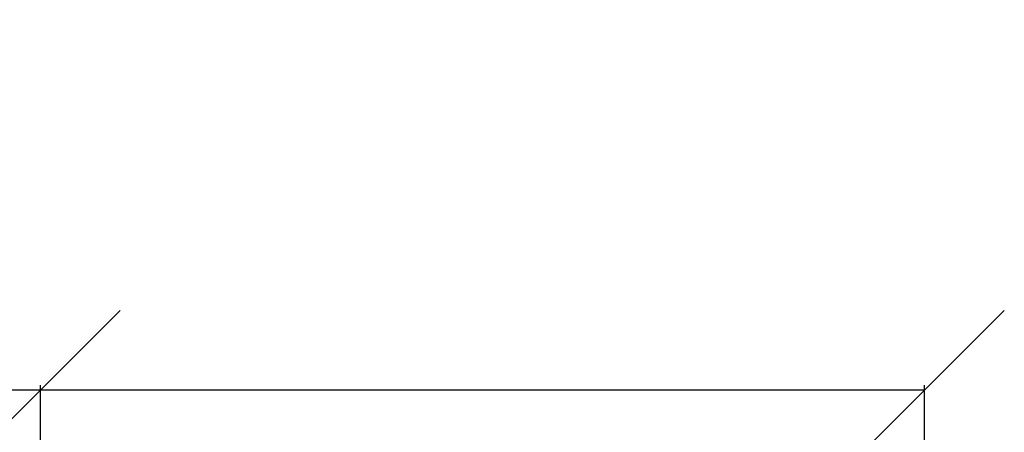
# Model space of a CAD drawing. Units: inches. Extents: x -1198 to -69, y -512 to 437.
# Tile 15 of 50: x -979 to -942, y 189 to 204. Entities that reach past the tile are written whole.
import ezdxf

# ---------------------------------------------------------------- set-up
doc = ezdxf.new("R2010")
doc.units = ezdxf.units.IN
doc.header["$MEASUREMENT"] = 0
doc.layers.add('A-ANNO-DIMS', color=2, linetype='Continuous', lineweight=18)
doc.styles.get("Standard").update_dxf_attribs({"font": 'arial.ttf'})
doc.dimstyles.get("Standard").update_dxf_attribs({"dimtxt": 6, "dimasz": 6, "dimexe": 0.18, "dimexo": 0.0625, "dimgap": 0.09, "dimtad": 0, "dimtih": 1, "dimtoh": 1, "dimdec": 0, "dimzin": 0, "dimdsep": 46, "dimlunit": 4, "dimtxsty": 'Standard', "dimblk": 'OBLIQUE', "dimcen": 0.09, "dimadec": 0, "dimazin": 0, "dimtfac": 1, "dimtdec": 0, "dimtofl": 0, "dimtmove": 0, "dimatfit": 3, "dimfxl": 1, "dimtolj": 1, "dimtzin": 0, "dimarcsym": 0})

# ---------------------------------------------------------------- blocks, each defined once
blk = doc.blocks.new('_Oblique')
at = {"color": 0, "linetype": 'ByBlock', "lineweight": -2}
blk.add_line((-0.5, -0.5), (0.5, 0.5), dxfattribs=at)
blk = doc.blocks.new('*D50')
at = {"layer": 'A-ANNO-DIMS', "color": 0, "lineweight": -2, "ltscale": 10, "transparency": 16777216}
for p, q in [((-978.462, 185.29), (-978.462, 190.403)), ((-945.163, 185.29), (-945.163, 190.403)), ((-978.462, 190.223), (-984.462, 190.223)), ((-945.163, 190.223), (-978.462, 190.223))]:
    blk.add_line(p, q, dxfattribs=at)
at = {"layer": 'DEFPOINTS', "color": 0, "ltscale": 10, "transparency": 16777216}
for p in [(-978.462, 190.223), (-978.462, 185.228), (-945.163, 185.228)]:
    blk.add_point(p, dxfattribs=at)
at = {"layer": 'A-ANNO-DIMS', "color": 0, "lineweight": -2, "ltscale": 10, "transparency": 16777216, "xscale": 6, "yscale": 6, "zscale": 6, "rotation": 180}
blk.add_blockref('_Oblique', (-978.462, 190.223), dxfattribs=at)
at = {"layer": 'A-ANNO-DIMS', "color": 0, "lineweight": -2, "ltscale": 10, "transparency": 16777216, "xscale": 6, "yscale": 6, "zscale": 6}
blk.add_blockref('_Oblique', (-945.163, 190.223), dxfattribs=at)
at = {"layer": 'A-ANNO-DIMS', "color": 0, "ltscale": 10, "transparency": 16777216, "insert": (-1009.24, 190.223), "char_height": 6, "attachment_point": 5}
blk.add_mtext('\\A1;HOB 33 TYP.', dxfattribs=at)

msp = doc.modelspace()

# ---------------------------------------------------------------- dimensions: what is measured, and where the dimension line sits
at = {"layer": 'A-ANNO-DIMS', "ltscale": 10}
dim = msp.add_linear_dim(base=(-978.4621, 190.2226), p1=(-945.1627, 185.2277), p2=(-978.4621, 185.2277), angle=180, text='HOB <> TYP.', dimstyle='Standard', override={"dimdec": 0, "dimlfac": 1, "dimrnd": 0, "dimzin": 0, "dimdsep": 46, "dimlunit": 2}, dxfattribs=at)
dim.commit()
dim.dimension.update_dxf_attribs({"geometry": '*D50', "text_midpoint": (-1009.2397, 190.2226)})

doc.saveas('drawing.dxf')
